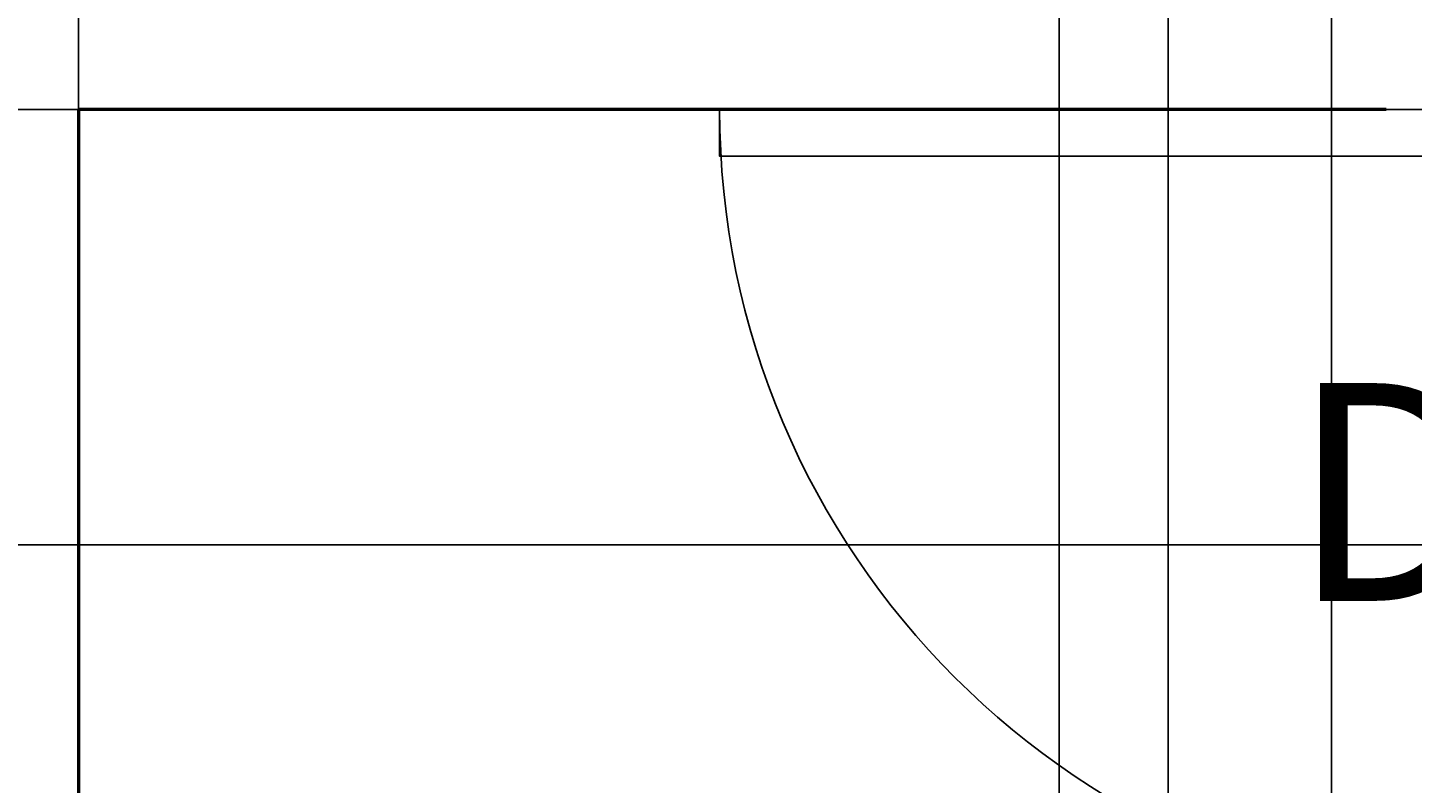
# Model space of a CAD drawing. Units: inches. Extents: x 37 to 824, y -700 to 234.
# Tile 47 of 77: x 168 to 219, y 50 to 78. Entities that reach past the tile are written whole.
import ezdxf

# ---------------------------------------------------------------- set-up
doc = ezdxf.new("R2010")
doc.units = ezdxf.units.IN
doc.header["$MEASUREMENT"] = 0
for name, color, linetype, lineweight in [('A-ANNO-DIMS', 2, 'Continuous', 18), ('A-ANNO-TEXT', 7, 'Continuous', 18), ('A-DOOR', 4, 'Continuous', 25), ('A-WALL', 2, 'Continuous', 50)]:
    doc.layers.add(name, color=color, linetype=linetype, lineweight=lineweight)
doc.styles.get("Standard").update_dxf_attribs({"font": 'arial.ttf'})
doc.dimstyles.get("Standard").update_dxf_attribs({"dimtxt": 0.18, "dimasz": 0.18, "dimexe": 0.18, "dimexo": 0.0625, "dimgap": 0.09, "dimtad": 0, "dimtih": 1, "dimtoh": 1, "dimdec": 1, "dimzin": 0, "dimdsep": 46, "dimlunit": 4, "dimtxsty": 'Standard', "dimcen": 0.09, "dimadec": 0, "dimazin": 0, "dimtfac": 1, "dimtdec": 1, "dimtofl": 0, "dimtmove": 0, "dimatfit": 3, "dimfxl": 1, "dimtolj": 1, "dimtzin": 0, "dimarcsym": 0})

# ---------------------------------------------------------------- blocks, each defined once
blk = doc.blocks.new('*U6')
for p, q in [((-750, 0), (-750, -100)), ((0, 0), (0, -100))]:
    blk.add_line(p, q)
blk.add_lwpolyline([(0, 0), (0, 750), (-43.75, 750), (-43.75, 0)], close=True)
blk.add_arc((0, 0), 750, 90, 180)
blk = doc.blocks.new('*D61')
at = {"layer": 'A-ANNO-DIMS', "color": 0, "lineweight": -2, "ltscale": 0.5, "transparency": 16777216}
for p, q in [((419.015, 75.09), (78.159, 75.09)), ((78.339, 74.91), (78.339, 67.271)), ((78.339, 59.27), (78.339, 66.91)), ((419.015, 59.09), (78.159, 59.09))]:
    blk.add_line(p, q, dxfattribs=at)
at = {"layer": 'A-ANNO-DIMS', "color": 0, "ltscale": 0.5, "transparency": 16777216}
for points in [[(78.309, 74.91), (78.369, 74.91), (78.339, 75.09)], [(78.309, 59.27), (78.369, 59.27), (78.339, 59.09)]]:
    blk.add_solid(points, dxfattribs=at)
at = {"layer": 'Defpoints', "color": 0, "ltscale": 0.5, "transparency": 16777216}
for p in [(419.077, 75.09), (78.339, 59.09), (419.077, 59.09)]:
    blk.add_point(p, dxfattribs=at)
at = {"layer": 'A-ANNO-DIMS', "color": 0, "ltscale": 0.5, "transparency": 16777216, "insert": (78.339, 67.09), "char_height": 0.18, "attachment_point": 5}
blk.add_mtext('\\A1;1\'-4"', dxfattribs=at)
blk = doc.blocks.new('*D84')
at = {"layer": 'A-ANNO-DIMS', "color": 0, "lineweight": -2, "ltscale": 0.5, "transparency": 16777216}
for p, q in [((170.077, -265.847), (170.077, 234.17)), ((170.257, 233.99), (189.748, 233.99)), ((209.897, 233.99), (190.406, 233.99)), ((210.077, -265.847), (210.077, 234.17))]:
    blk.add_line(p, q, dxfattribs=at)
at = {"layer": 'A-ANNO-DIMS', "color": 0, "ltscale": 0.5, "transparency": 16777216}
for points in [[(170.257, 234.02), (170.257, 233.96), (170.077, 233.99)], [(209.897, 234.02), (209.897, 233.96), (210.077, 233.99)]]:
    blk.add_solid(points, dxfattribs=at)
at = {"layer": 'Defpoints', "color": 0, "ltscale": 0.5, "transparency": 16777216}
for p in [(210.077, 233.99), (170.077, -265.91), (210.077, -265.91)]:
    blk.add_point(p, dxfattribs=at)
at = {"layer": 'A-ANNO-DIMS', "color": 0, "ltscale": 0.5, "transparency": 16777216, "insert": (190.077, 233.99), "char_height": 0.18, "attachment_point": 5}
blk.add_mtext('\\A1;3\'-4"', dxfattribs=at)
blk = doc.blocks.new('*D85')
at = {"layer": 'A-ANNO-DIMS', "color": 0, "lineweight": -2, "ltscale": 0.5, "transparency": 16777216}
for p, q in [((170.077, -356.847), (170.077, 234.17)), ((170.257, 233.99), (187.748, 233.99)), ((205.897, 233.99), (188.406, 233.99)), ((206.077, -356.847), (206.077, 234.17))]:
    blk.add_line(p, q, dxfattribs=at)
at = {"layer": 'A-ANNO-DIMS', "color": 0, "ltscale": 0.5, "transparency": 16777216}
for points in [[(170.257, 234.02), (170.257, 233.96), (170.077, 233.99)], [(205.897, 234.02), (205.897, 233.96), (206.077, 233.99)]]:
    blk.add_solid(points, dxfattribs=at)
at = {"layer": 'Defpoints', "color": 0, "ltscale": 0.5, "transparency": 16777216}
for p in [(206.077, 233.99), (170.077, -356.91), (206.077, -356.91)]:
    blk.add_point(p, dxfattribs=at)
at = {"layer": 'A-ANNO-DIMS', "color": 0, "ltscale": 0.5, "transparency": 16777216, "insert": (188.077, 233.99), "char_height": 0.18, "attachment_point": 5}
blk.add_mtext('\\A1;3\'-0"', dxfattribs=at)
blk = doc.blocks.new('*D86')
at = {"layer": 'A-ANNO-DIMS', "color": 0, "lineweight": -2, "ltscale": 0.5, "transparency": 16777216}
for p, q in [((206.077, -356.847), (206.077, 234.17)), ((206.257, 233.99), (210.678, 233.99)), ((215.897, 233.99), (211.476, 233.99)), ((216.077, -356.847), (216.077, 234.17))]:
    blk.add_line(p, q, dxfattribs=at)
at = {"layer": 'A-ANNO-DIMS', "color": 0, "ltscale": 0.5, "transparency": 16777216}
for points in [[(206.257, 234.02), (206.257, 233.96), (206.077, 233.99)], [(215.897, 234.02), (215.897, 233.96), (216.077, 233.99)]]:
    blk.add_solid(points, dxfattribs=at)
at = {"layer": 'Defpoints', "color": 0, "ltscale": 0.5, "transparency": 16777216}
for p in [(216.077, 233.99), (206.077, -356.91), (216.077, -356.91)]:
    blk.add_point(p, dxfattribs=at)
at = {"layer": 'A-ANNO-DIMS', "color": 0, "ltscale": 0.5, "transparency": 16777216, "insert": (211.077, 233.99), "char_height": 0.18, "attachment_point": 5}
blk.add_mtext('\\A1;0\'-10"', dxfattribs=at)
blk = doc.blocks.new('*D87')
at = {"layer": 'A-ANNO-DIMS', "color": 0, "lineweight": -2, "ltscale": 0.5, "transparency": 16777216}
for p, q in [((216.077, -356.847), (216.077, 234.17)), ((216.257, 233.99), (255.747, 233.99)), ((295.897, 233.99), (256.407, 233.99)), ((296.077, -356.847), (296.077, 234.17))]:
    blk.add_line(p, q, dxfattribs=at)
at = {"layer": 'A-ANNO-DIMS', "color": 0, "ltscale": 0.5, "transparency": 16777216}
for points in [[(216.257, 234.02), (216.257, 233.96), (216.077, 233.99)], [(295.897, 234.02), (295.897, 233.96), (296.077, 233.99)]]:
    blk.add_solid(points, dxfattribs=at)
at = {"layer": 'Defpoints', "color": 0, "ltscale": 0.5, "transparency": 16777216}
for p in [(296.077, 233.99), (216.077, -356.91), (296.077, -356.91)]:
    blk.add_point(p, dxfattribs=at)
at = {"layer": 'A-ANNO-DIMS', "color": 0, "ltscale": 0.5, "transparency": 16777216, "insert": (256.077, 233.99), "char_height": 0.18, "attachment_point": 5}
blk.add_mtext('\\A1;6\'-8"', dxfattribs=at)

msp = doc.modelspace()

# ---------------------------------------------------------------- linework, layer by layer
at = {"layer": 'A-WALL'}
for p, q in [((170.077, 75.09), (170.077, -2.91)), ((218.077, 75.09), (170.077, 75.09))]:
    msp.add_line(p, q, dxfattribs=at)

# ---------------------------------------------------------------- block references
at = {"layer": 'A-DOOR', "xscale": 0.0393700787401575, "yscale": 0.0393700787401575, "zscale": 0.0393700787401575, "rotation": 90}
msp.add_blockref('*U6', (223.14, 75.09), dxfattribs=at)

# ---------------------------------------------------------------- texts
at = {"layer": 'A-ANNO-TEXT'}
msp.add_text('D1', height=8, dxfattribs=at).set_placement((214.553, 57.037))

# ---------------------------------------------------------------- dimensions: what is measured, and where the dimension line sits
at = {"layer": 'A-ANNO-DIMS', "ltscale": 0.5}
for base, p1, p2, picture, middle in [((210.077, 233.99), (170.077, -265.91), (210.077, -265.91), '*D84', (190.077, 233.99)), ((206.077, 233.99), (170.077, -356.91), (206.077, -356.91), '*D85', (188.077, 233.99)), ((216.077, 233.99), (206.077, -356.91), (216.077, -356.91), '*D86', (211.077, 233.99)), ((296.077, 233.99), (216.077, -356.91), (296.077, -356.91), '*D87', (256.077, 233.99))]:
    dim = msp.add_linear_dim(base=base, p1=p1, p2=p2, dimstyle='Standard', override={"dimdec": 1, "dimlfac": 1, "dimrnd": 0, "dimzin": 1, "dimdsep": 46, "dimlunit": 4, "dimfrac": 2}, dxfattribs=at)
    dim.commit()
    dim.dimension.update_dxf_attribs({"geometry": picture, "text_midpoint": middle})
dim = msp.add_linear_dim(base=(78.339, 59.09), p1=(419.077, 75.09), p2=(419.077, 59.09), angle=90, dimstyle='Standard', override={"dimdec": 1, "dimlfac": 1, "dimrnd": 0, "dimzin": 1, "dimdsep": 46, "dimlunit": 4, "dimfrac": 2}, dxfattribs=at)
dim.commit()
dim.dimension.update_dxf_attribs({"geometry": '*D61', "text_midpoint": (78.339, 67.09)})

doc.saveas('drawing.dxf')
